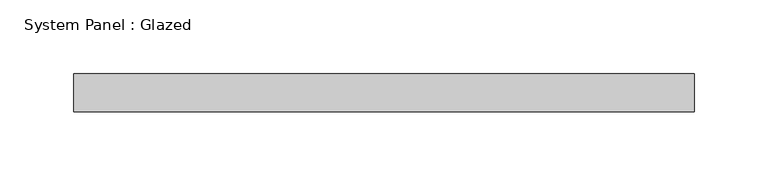
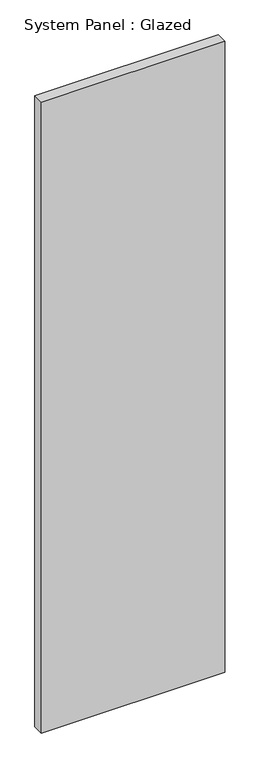
"""IFC4 building model written with IfcOpenShell, lengths in millimetres: plate geometry, System Panel : Glazed."""

from ifc_helpers import new_model, si_unit, origin, origin_with_axes, place, context, project, spatial, polyline, outline, extrude, source, transform, mapped, element, save


def system_panel_glazed_49ff1c72(model_context):
    return source(origin(), model_context, "Body", "SweptSolid", [
        extrude(outline(polyline([(209.55, 19.05), (-209.55, 19.05), (-209.55, 44.45), (209.55, 44.45), (209.55, 19.05)])), origin_with_axes(), (0.0, 0.0, 1.0), 1524.0),
    ])


if __name__ == "__main__":
    model = new_model("IFC4")
    model_context = context("Model", 3, world=origin())
    ifc_project = project(units=[si_unit("LENGTHUNIT", "METRE", prefix="MILLI")], contexts=[model_context])
    site = spatial("IfcSite", under=ifc_project)
    building = spatial("IfcBuilding", under=site)
    placement = place(None, origin())
    system_panel_glazed_shape = system_panel_glazed_49ff1c72(model_context)
    element("IfcPlate", 1, ObjectType="System Panel : Glazed", at=placement, inside=building, context=model_context, shape_type="MappedRepresentation", body=[
        mapped(system_panel_glazed_shape, transform((0.0, 0.0, 0.0), x_axis=(1.0, 0.0, 0.0), y_axis=(0.0, 1.0, 0.0), z_axis=(0.0, 0.0, 1.0))),
    ])
    save(model, "model.ifc")

# Revit data of these elements
# Type "System Panel : Glazed"
#   Construction Type Id = "GSP4R"
#   Analytic Construction = "1/8 in Pilkington single glazing"
#   Visual Light Transmittance = 0.9
#   Solar Heat Gain Coefficient = 0.86
#   Heat Transfer Coefficient (U) = 1.18115 BTU/(h·ft²·°F)
#   Define Thermal Properties by = 1
# Element 1 (IfcPlate, "System Panel : Glazed")
#   Materials on its faces: "Glass"
# Materials
#   "Glass": class "Glass", colour RGB 0 128 192, transparency 0.75, Description = "Soda Lime Glass", Cost = 0
